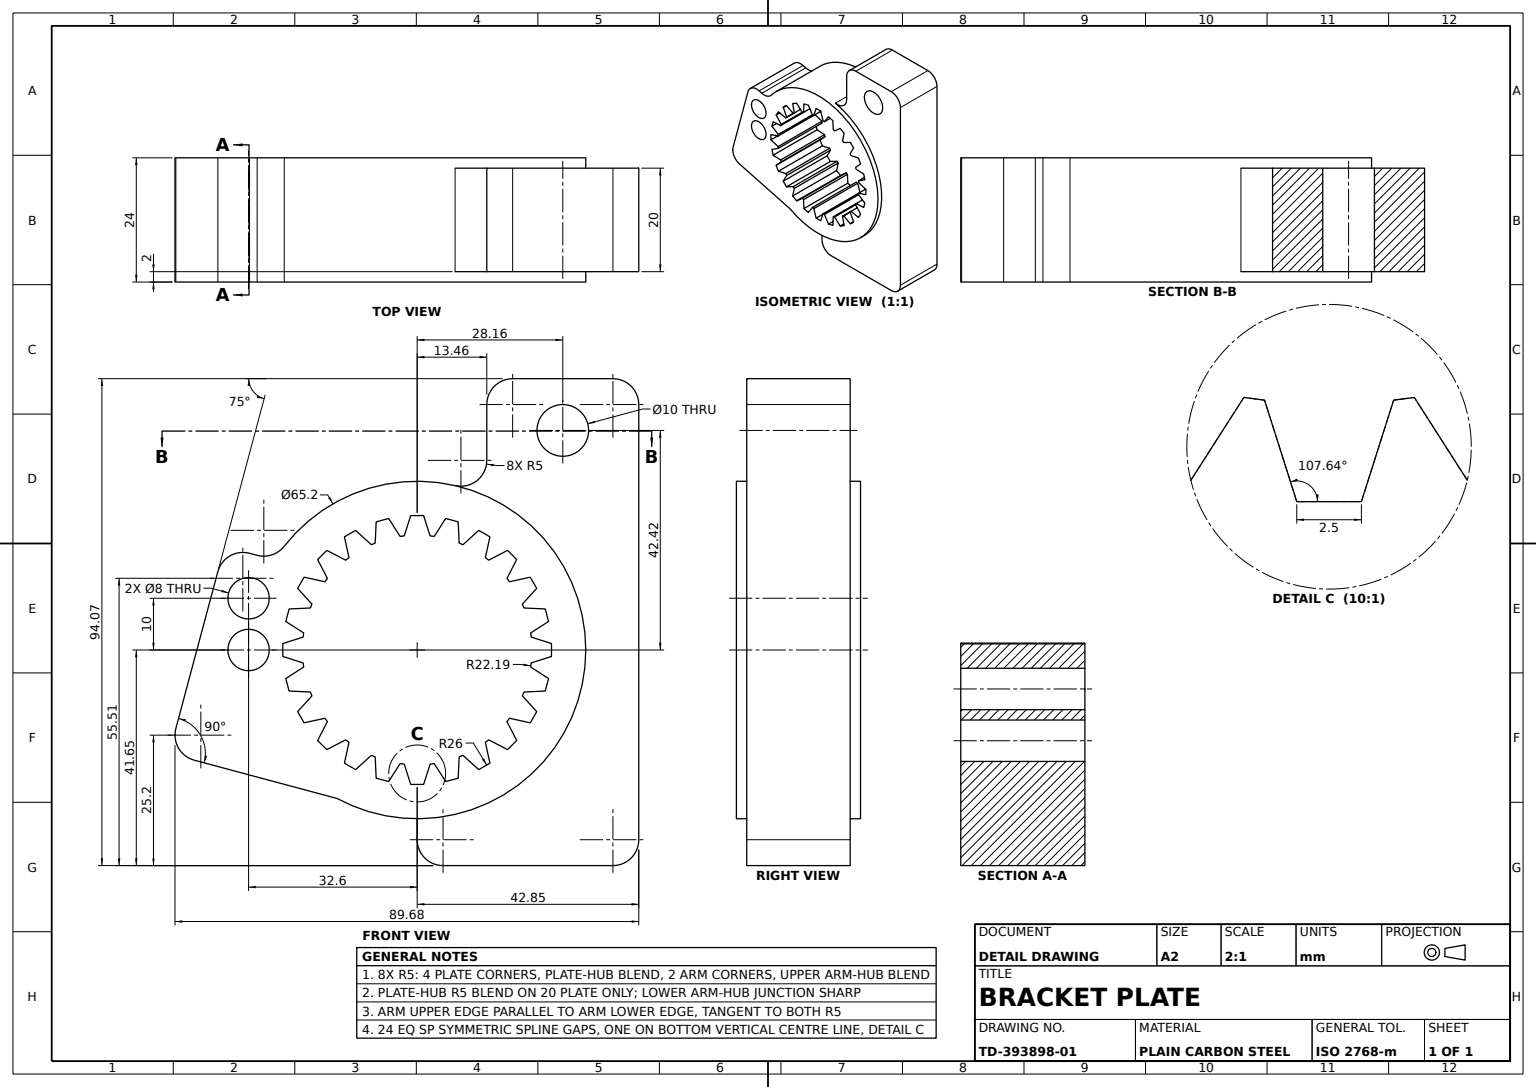
from build123d import *

# Parameters (mm, degrees)
SPLINED_HUB_PROFILE_R   = 32.6
SPLINED_HUB_24T_DEPTH   = 12
MOUNTING_FLANGE_DEPTH   = 10
SIDE_LUG_DEPTH          = 12
LUG_HOLE_PROFILE_R      = 5
LUG_HOLE_10_DEPTH       = 10
LUG_FILLET_R5_R         = 5
FLANGE_HOLES_PROFILE_R  = 4
FLANGE_HOLES_2X_8_DEPTH = 74.654745929
FLANGE_SLOT_PROFILE_R   = 4
FLANGE_SLOT_DEPTH       = 12


with BuildPart() as part:
    # Splined Hub Profile → Splined Hub 24T (new, symmetric)
    with BuildSketch(Plane.XY):
        Circle(SPLINED_HUB_PROFILE_R)
        with BuildLine():
            ThreePointArc((25.969951923, 1.249638793), (25.992486895, 0.625), (26, 0))
            ThreePointArc((26, 0), (25.992486895, -0.625), (25.969951923, -1.249638793))
            Line((25.969951923, -1.249638793), (22.049170798, -2.496030275))
            ThreePointArc((22.049170798, -2.496030275), (22.000161474, -2.896376205), (21.943883694, -3.295765225))
            Line((21.943883694, -3.295765225), (25.408477589, -5.514459774))
            ThreePointArc((25.408477589, -5.514459774), (25.114071484, -6.729295173), (24.761616951, -7.928576542))
            Line((24.761616951, -7.928576542), (20.651843349, -8.117725437))
            ThreePointArc((20.651843349, -8.117725437), (20.500886826, -8.491745364), (20.343157181, -8.862959772))
            Line((20.343157181, -8.862959772), (23.115457497, -11.902757021))
            ThreePointArc((23.115457497, -11.902757021), (22.516660498, -13), (21.865818704, -14.067194902))
            Line((21.865818704, -14.067194902), (17.847126905, -13.186211026))
            ThreePointArc((17.847126905, -13.186211026), (17.604510621, -13.50841611), (17.356078124, -13.826158257))
            Line((17.356078124, -13.826158257), (19.247157176, -17.479901047))
            ThreePointArc((19.247157176, -17.479901047), (18.384776311, -18.384776311), (17.479901047, -19.247157176))
            Line((17.479901047, -19.247157176), (13.826158257, -17.356078124))
            ThreePointArc((13.826158257, -17.356078124), (13.50841611, -17.604510621), (13.186211026, -17.847126905))
            Line((13.186211026, -17.847126905), (14.067194902, -21.865818704))
            ThreePointArc((14.067194902, -21.865818704), (13, -22.516660498), (11.902757021, -23.115457497))
            Line((11.902757021, -23.115457497), (8.862959772, -20.343157181))
            ThreePointArc((8.862959772, -20.343157181), (8.491745364, -20.500886826), (8.117725437, -20.651843349))
            Line((8.117725437, -20.651843349), (7.928576542, -24.761616951))
            ThreePointArc((7.928576542, -24.761616951), (6.729295173, -25.114071484), (5.514459774, -25.408477589))
            Line((5.514459774, -25.408477589), (3.295765225, -21.943883694))
            ThreePointArc((3.295765225, -21.943883694), (2.896376205, -22.000161474), (2.496030275, -22.049170798))
            Line((2.496030275, -22.049170798), (1.249638793, -25.969951923))
            ThreePointArc((1.249638793, -25.969951923), (0, -26), (-1.249638793, -25.969951923))
            Line((-1.249638793, -25.969951923), (-2.496030275, -22.049170798))
            ThreePointArc((-2.496030275, -22.049170798), (-2.896376205, -22.000161474), (-3.295765225, -21.943883694))
            Line((-3.295765225, -21.943883694), (-5.514459774, -25.408477589))
            ThreePointArc((-5.514459774, -25.408477589), (-6.729295173, -25.114071484), (-7.928576542, -24.761616951))
            Line((-7.928576542, -24.761616951), (-8.117725437, -20.651843349))
            ThreePointArc((-8.117725437, -20.651843349), (-8.491745364, -20.500886826), (-8.862959772, -20.343157181))
            Line((-8.862959772, -20.343157181), (-11.902757021, -23.115457497))
            ThreePointArc((-11.902757021, -23.115457497), (-13, -22.516660498), (-14.067194902, -21.865818704))
            Line((-14.067194902, -21.865818704), (-13.186211026, -17.847126905))
            ThreePointArc((-13.186211026, -17.847126905), (-13.50841611, -17.604510621), (-13.826158257, -17.356078124))
            Line((-13.826158257, -17.356078124), (-17.479901047, -19.247157176))
            ThreePointArc((-17.479901047, -19.247157176), (-18.384776311, -18.384776311), (-19.247157176, -17.479901047))
            Line((-19.247157176, -17.479901047), (-17.356078124, -13.826158257))
            ThreePointArc((-17.356078124, -13.826158257), (-17.604510621, -13.50841611), (-17.847126905, -13.186211026))
            Line((-17.847126905, -13.186211026), (-21.865818704, -14.067194902))
            ThreePointArc((-21.865818704, -14.067194902), (-22.516660498, -13), (-23.115457497, -11.902757021))
            Line((-23.115457497, -11.902757021), (-20.343157181, -8.862959772))
            ThreePointArc((-20.343157181, -8.862959772), (-20.500886826, -8.491745364), (-20.651843349, -8.117725437))
            Line((-20.651843349, -8.117725437), (-24.761616951, -7.928576542))
            ThreePointArc((-24.761616951, -7.928576542), (-25.114071484, -6.729295173), (-25.408477589, -5.514459774))
            Line((-25.408477589, -5.514459774), (-21.943883694, -3.295765225))
            ThreePointArc((-21.943883694, -3.295765225), (-22.000161474, -2.896376205), (-22.049170798, -2.496030275))
            Line((-22.049170798, -2.496030275), (-25.969951923, -1.249638793))
            ThreePointArc((-25.969951923, -1.249638793), (-26, 0), (-25.969951923, 1.249638793))
            Line((-25.969951923, 1.249638793), (-22.049170798, 2.496030275))
            ThreePointArc((-22.049170798, 2.496030275), (-22.000161474, 2.896376205), (-21.943883694, 3.295765225))
            Line((-21.943883694, 3.295765225), (-25.408477589, 5.514459774))
            ThreePointArc((-25.408477589, 5.514459774), (-25.114071484, 6.729295173), (-24.761616951, 7.928576542))
            Line((-24.761616951, 7.928576542), (-20.651843349, 8.117725437))
            ThreePointArc((-20.651843349, 8.117725437), (-20.500886826, 8.491745364), (-20.343157181, 8.862959772))
            Line((-20.343157181, 8.862959772), (-23.115457497, 11.902757021))
            ThreePointArc((-23.115457497, 11.902757021), (-22.516660498, 13), (-21.865818704, 14.067194902))
            Line((-21.865818704, 14.067194902), (-17.847126905, 13.186211026))
            ThreePointArc((-17.847126905, 13.186211026), (-17.604510621, 13.50841611), (-17.356078124, 13.826158257))
            Line((-17.356078124, 13.826158257), (-19.247157176, 17.479901047))
            ThreePointArc((-19.247157176, 17.479901047), (-18.384776311, 18.384776311), (-17.479901047, 19.247157176))
            Line((-17.479901047, 19.247157176), (-13.826158257, 17.356078124))
            ThreePointArc((-13.826158257, 17.356078124), (-13.50841611, 17.604510621), (-13.186211026, 17.847126905))
            Line((-13.186211026, 17.847126905), (-14.067194902, 21.865818704))
            ThreePointArc((-14.067194902, 21.865818704), (-13, 22.516660498), (-11.902757021, 23.115457497))
            Line((-11.902757021, 23.115457497), (-8.862959772, 20.343157181))
            ThreePointArc((-8.862959772, 20.343157181), (-8.491745364, 20.500886826), (-8.117725437, 20.651843349))
            Line((-8.117725437, 20.651843349), (-7.928576542, 24.761616951))
            ThreePointArc((-7.928576542, 24.761616951), (-6.729295173, 25.114071484), (-5.514459774, 25.408477589))
            Line((-5.514459774, 25.408477589), (-3.295765225, 21.943883694))
            ThreePointArc((-3.295765225, 21.943883694), (-2.896376205, 22.000161474), (-2.496030275, 22.049170798))
            Line((-2.496030275, 22.049170798), (-1.249638793, 25.969951923))
            ThreePointArc((-1.249638793, 25.969951923), (0, 26), (1.249638793, 25.969951923))
            Line((1.249638793, 25.969951923), (2.496030275, 22.049170798))
            ThreePointArc((2.496030275, 22.049170798), (2.896376205, 22.000161474), (3.295765225, 21.943883694))
            Line((3.295765225, 21.943883694), (5.514459774, 25.408477589))
            ThreePointArc((5.514459774, 25.408477589), (6.729295173, 25.114071484), (7.928576542, 24.761616951))
            Line((7.928576542, 24.761616951), (8.117725437, 20.651843349))
            ThreePointArc((8.117725437, 20.651843349), (8.491745364, 20.500886826), (8.862959772, 20.343157181))
            Line((8.862959772, 20.343157181), (11.902757021, 23.115457497))
            ThreePointArc((11.902757021, 23.115457497), (13, 22.516660498), (14.067194902, 21.865818704))
            Line((14.067194902, 21.865818704), (13.186211026, 17.847126905))
            ThreePointArc((13.186211026, 17.847126905), (13.50841611, 17.604510621), (13.826158257, 17.356078124))
            Line((13.826158257, 17.356078124), (17.479901047, 19.247157176))
            ThreePointArc((17.479901047, 19.247157176), (18.384776311, 18.384776311), (19.247157176, 17.479901047))
            Line((19.247157176, 17.479901047), (17.356078124, 13.826158257))
            ThreePointArc((17.356078124, 13.826158257), (17.604510621, 13.50841611), (17.847126905, 13.186211026))
            Line((17.847126905, 13.186211026), (21.865818704, 14.067194902))
            ThreePointArc((21.865818704, 14.067194902), (22.516660498, 13), (23.115457497, 11.902757021))
            Line((23.115457497, 11.902757021), (20.343157181, 8.862959772))
            ThreePointArc((20.343157181, 8.862959772), (20.500886826, 8.491745364), (20.651843349, 8.117725437))
            Line((20.651843349, 8.117725437), (24.761616951, 7.928576542))
            ThreePointArc((24.761616951, 7.928576542), (25.114071484, 6.729295173), (25.408477589, 5.514459774))
            Line((25.408477589, 5.514459774), (21.943883694, 3.295765225))
            ThreePointArc((21.943883694, 3.295765225), (22.000161474, 2.896376205), (22.049170798, 2.496030275))
            Line((22.049170798, 2.496030275), (25.969951923, 1.249638793))
        make_face(mode=Mode.SUBTRACT)
    extrude(amount=SPLINED_HUB_24T_DEPTH, both=True)

    # Mounting Flange Profile → Mounting Flange (add, symmetric)
    with BuildSketch(Plane.XY):
        with BuildLine():
            Line((42.85, 0), (42.85, -36.65))
            ThreePointArc((42.85, -36.65), (41.385533906, -40.185533906), (37.85, -41.65))
            Line((37.85, -41.65), (5, -41.65))
            ThreePointArc((5, -41.65), (1.464466094, -40.185533906), (0, -36.65))
            Line((0, -36.65), (0, -32.6))
            ThreePointArc((0, -32.6), (32.390349794, -3.691238309), (7.335, 31.76409569))
            ThreePointArc((7.335, 31.76409569), (11.572474899, 32.722770547), (13.46, 36.635889507))
            Line((13.46, 36.635889507), (13.46, 47.42))
            ThreePointArc((13.46, 47.42), (14.924466094, 50.955533906), (18.46, 52.42))
            Line((18.46, 52.42), (37.85, 52.42))
            ThreePointArc((37.85, 52.42), (41.385533906, 50.955533906), (42.85, 47.42))
            Line((42.85, 47.42), (42.85, 0))
        make_face()
    extrude(amount=MOUNTING_FLANGE_DEPTH, both=True)

    # Side Lug Profile → Side Lug (add, symmetric)
    with BuildSketch(Plane.XY):
        with BuildLine():
            Line((-37.246328052, 19.980175717), (-47.954966043, -19.985005346))
            Line((-47.954966043, -19.985005346), (-15.493199502, -28.683109475))
            ThreePointArc((-15.493199502, -28.683109475), (-31.533730192, -8.269453439), (-27.575166089, 17.388795679))
            Line((-27.575166089, 17.388795679), (-37.246328052, 19.980175717))
        make_face()
    extrude(amount=SIDE_LUG_DEPTH, both=True)

    # Lug Hole Profile → Lug Hole Ø10 (cut, symmetric)
    with BuildSketch(Plane.XY):
        with Locations((28.155, 42.42)):
            Circle(LUG_HOLE_PROFILE_R)
    extrude(amount=LUG_HOLE_10_DEPTH, both=True, mode=Mode.SUBTRACT)

    # Lug Fillet R5
    lug_fillet_r5_edges = [part.edges().sort_by_distance(p)[0] for p in [
        (-27.575166089, 17.388795679, 0),
        (-37.246328052, 19.980175717, 0),
        (-47.954966043, -19.985005346, 0),
    ]]
    fillet(lug_fillet_r5_edges, radius=LUG_FILLET_R5_R)

    # Flange Holes Profile → Flange Holes 2xØ8 (cut, through all)
    with BuildSketch(Plane.XY.offset(10)):
        with Locations((-32.6, 0)):
            Circle(FLANGE_HOLES_PROFILE_R)
    extrude(amount=-FLANGE_HOLES_2X_8_DEPTH, mode=Mode.SUBTRACT)

    # Flange Slot Profile → Flange Slot (cut, symmetric)
    with BuildSketch(Plane.XY):
        with Locations((-32.6, 0)):
            Circle(FLANGE_SLOT_PROFILE_R)
        with Locations((-32.6, 10)):
            Circle(FLANGE_SLOT_PROFILE_R)
    extrude(amount=FLANGE_SLOT_DEPTH, both=True, mode=Mode.SUBTRACT)


solid = part.part
